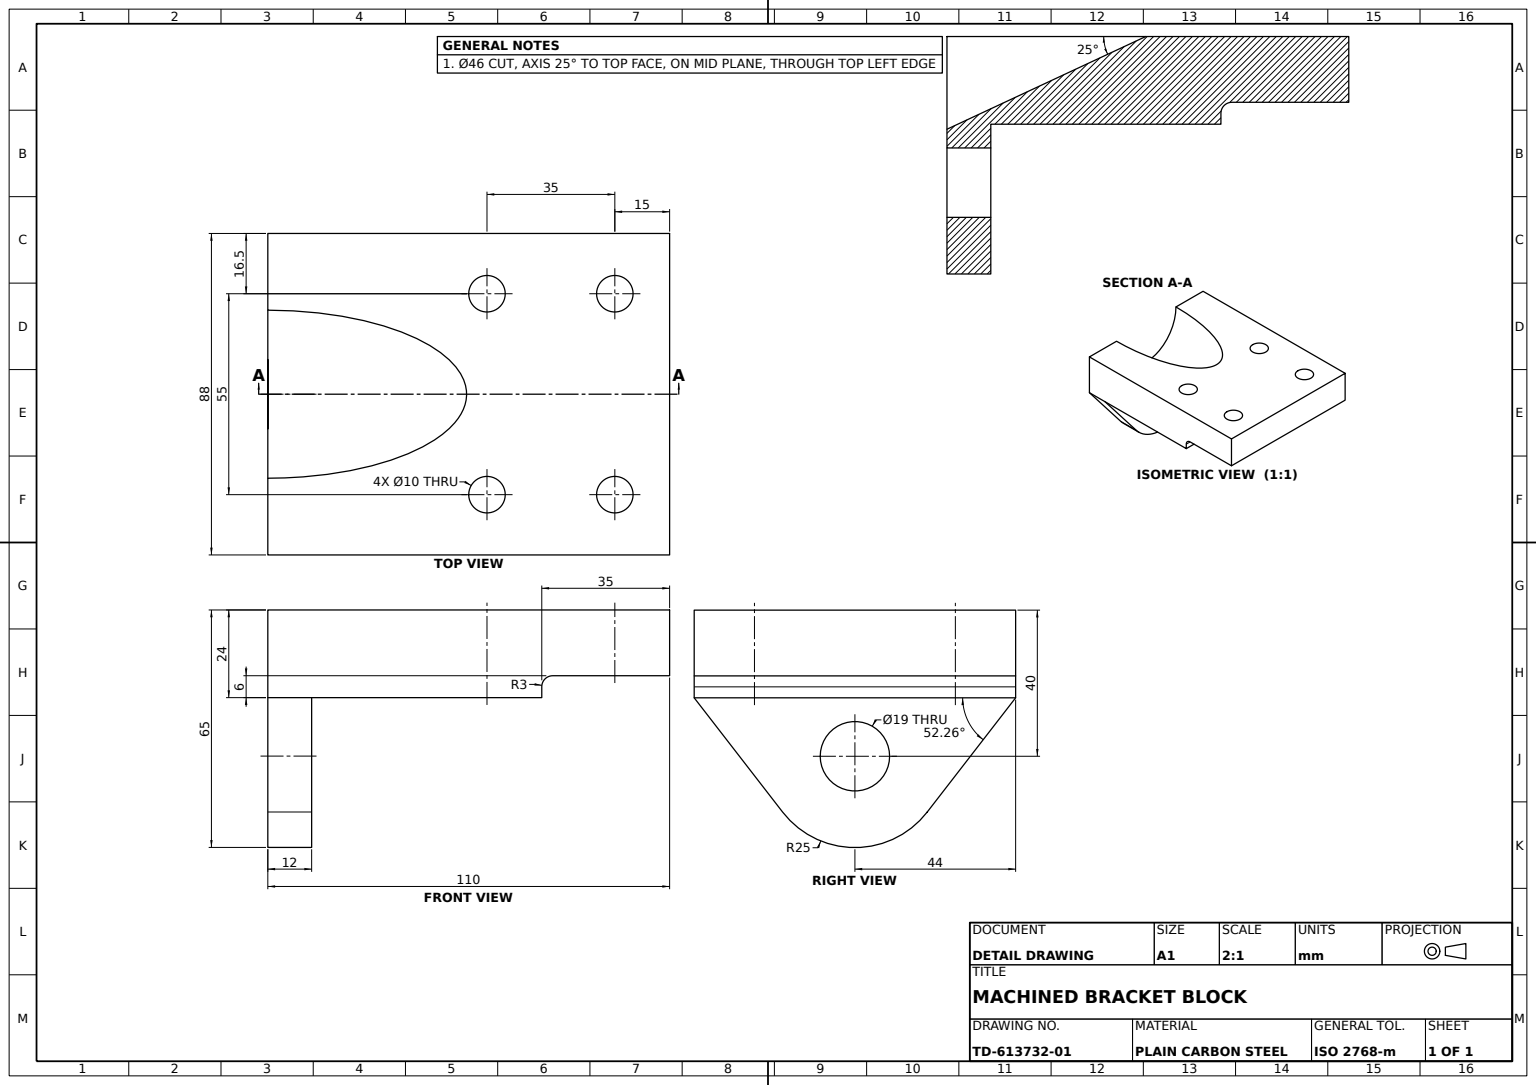
from build123d import *

# Parameters (mm, degrees)
BODY_PROFILE_SKETCH_R          = 25
BODY_PROFILE_SKETCH_R_2        = 9.5
BRACKET_BODY_EXTRUDE_110_DEPTH = 110
THROUGH_SLOT_CUT_DEPTH         = 110
ANGLED_BORE_SKETCH_46_R        = 23
ANGLED_BORE_46_DEPTH           = 55
MOUNTING_HOLES_SKETCH_R        = 5
MOUNTING_HOLES_4X_10_DEPTH     = 55


with BuildPart() as part:
    # Body Profile Sketch → Bracket Body Extrude 110 (new body)
    # profile 1 of 2: a face of its own
    with BuildSketch(Plane.XY):
        with BuildLine():
            Line((44, 0), (-44, 0))
            Line((-44, 0), (-44, -24))
            Line((-44, -24), (-19.769224603, -55.302867659))
            ThreePointArc((-19.769224603, -55.302867659), (-8.086080167, -16.343810376), (25, -40))
            ThreePointArc((25, -40), (23.656189624, -48.086080167), (19.769224603, -55.302867659))
            Line((19.769224603, -55.302867659), (44, -24))
            Line((44, -24), (44, 0))
        make_face()
    # profile 2 of 2: a face of its own
    with BuildSketch(Plane.XY):
        with Locations((0, -40)):
            Circle(BODY_PROFILE_SKETCH_R)
        with Locations((0, -40)):
            Circle(BODY_PROFILE_SKETCH_R_2, mode=Mode.SUBTRACT)
    extrude(amount=-BRACKET_BODY_EXTRUDE_110_DEPTH)

    # Through Slot Sketch → Through Slot Cut (cut)
    with BuildSketch(Plane(origin=(44, 0, 0), x_dir=(0, 0, -1), z_dir=(1, 0, 0))):
        with BuildLine():
            Line((12, -76.359959314), (12, -24))
            Line((12, -24), (75, -24))
            Line((75, -24), (75, -21))
            ThreePointArc((75, -21), (75.878679656, -18.878679656), (78, -18))
            Line((78, -18), (121.77138992, -18))
            Line((121.77138992, -18), (130.17802, -76.359959314))
            Line((130.17802, -76.359959314), (12, -76.359959314))
        make_face()
    extrude(amount=-THROUGH_SLOT_CUT_DEPTH, mode=Mode.SUBTRACT)

    # Angled Bore Sketch Ø46 → Angled Bore Ø46 (cut, symmetric)
    with BuildSketch(Plane(origin=(0, 0, 0), x_dir=(-1, 0, 0), z_dir=(0, 0.4226182617406939, -0.9063077870366526))):
        Circle(ANGLED_BORE_SKETCH_46_R)
    extrude(amount=ANGLED_BORE_46_DEPTH, both=True, mode=Mode.SUBTRACT)

    # Mounting Holes Sketch → Mounting Holes 4xØ10 (cut, symmetric)
    with BuildSketch(Plane(origin=(0, 0, 0), x_dir=(1, 0, 0), z_dir=(0, 1, 0))):
        with Locations(Location((-27.5, 95, 0), (0, 0, 180))):
            Circle(MOUNTING_HOLES_SKETCH_R)
        with Locations(Location((-27.5, 60, 0), (0, 0, 180))):
            Circle(MOUNTING_HOLES_SKETCH_R)
        with Locations(Location((27.5, 60, 0), (0, 0, 180))):
            Circle(MOUNTING_HOLES_SKETCH_R)
        with Locations(Location((27.5, 95, 0), (0, 0, 180))):
            Circle(MOUNTING_HOLES_SKETCH_R)
    extrude(amount=MOUNTING_HOLES_4X_10_DEPTH, both=True, mode=Mode.SUBTRACT)


solid = part.part
